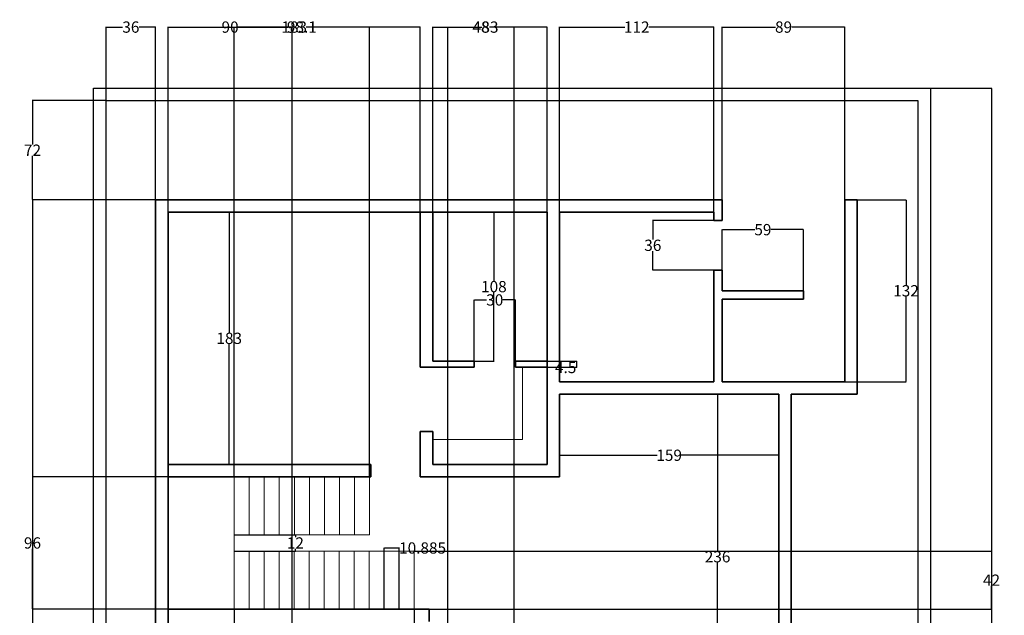
# Model space of a CAD drawing. Units: inches. Extents: x -254 to 1961, y 86 to 3025.
# Tile 6 of 6: x 1247 to 1961, y 2593 to 3025. Entities that reach past the tile are written whole.
import ezdxf

# ---------------------------------------------------------------- set-up
doc = ezdxf.new("R2010")
doc.units = ezdxf.units.IN
doc.header["$MEASUREMENT"] = 0
for name, color, linetype, lineweight in [('A-ANNO-DIMS', 2, 'Continuous', 18), ('C-SITE-WALL', 8, 'Continuous', 30), ('KITCHEN', 9, 'Continuous', 18), ('STAIRCASE', 212, 'Continuous', 18), ('WALLS', 255, 'Continuous', 35)]:
    doc.layers.add(name, color=color, linetype=linetype, lineweight=lineweight)
doc.styles.get("Standard").update_dxf_attribs({"font": 'arial.ttf'})
doc.dimstyles.get("Standard").update_dxf_attribs({"dimtxt": 8.18, "dimasz": 0.18, "dimexe": 0.18, "dimexo": 0.0625, "dimgap": 0.09, "dimtad": 0, "dimtih": 1, "dimtoh": 1, "dimdec": 1, "dimzin": 0, "dimdsep": 46, "dimlunit": 3, "dimtxsty": 'Standard', "dimcen": 0.09, "dimadec": 0, "dimazin": 0, "dimtfac": 1, "dimtdec": 1, "dimtofl": 0, "dimtmove": 0, "dimatfit": 3, "dimfxl": 1, "dimtolj": 1, "dimtzin": 0, "dimarcsym": 0})

# ---------------------------------------------------------------- blocks, each defined once
blk = doc.blocks.new('*D72')
at = {"layer": 'A-ANNO-DIMS', "color": 0, "lineweight": -2, "transparency": 16777216}
for p, q in [((1907.43, 2975.46), (1951.9, 2975.46)), ((1951.72, 2975.28), (1951.72, 2539.72)), ((1951.72, 2095.64), (1951.72, 2531.19)), ((1907.43, 2095.46), (1951.9, 2095.46))]:
    blk.add_line(p, q, dxfattribs=at)
at = {"layer": 'A-ANNO-DIMS', "color": 0, "transparency": 16777216}
for points in [[(1951.69, 2975.28), (1951.75, 2975.28), (1951.72, 2975.46)], [(1951.69, 2095.64), (1951.75, 2095.64), (1951.72, 2095.46)]]:
    blk.add_solid(points, dxfattribs=at)
at = {"layer": 'Defpoints', "color": 0, "transparency": 16777216}
for p in [(1907.37, 2975.46), (1951.72, 2975.46), (1907.37, 2095.46)]:
    blk.add_point(p, dxfattribs=at)
at = {"layer": 'A-ANNO-DIMS', "color": 0, "transparency": 16777216, "insert": (1951.72, 2535.46), "char_height": 8.18, "attachment_point": 5}
blk.add_mtext('\\A1;880', dxfattribs=at)
blk = doc.blocks.new('*D74')
at = {"layer": 'A-ANNO-DIMS', "color": 0, "lineweight": -2, "transparency": 16777216}
for p, q in [((1345.31, 2894.46), (1255.84, 2894.46)), ((1256.02, 2894.28), (1256.02, 2521.71)), ((1256.02, 2140.64), (1256.02, 2513.21)), ((1345.31, 2140.46), (1255.84, 2140.46))]:
    blk.add_line(p, q, dxfattribs=at)
at = {"layer": 'A-ANNO-DIMS', "color": 0, "transparency": 16777216}
for points in [[(1255.99, 2894.28), (1256.05, 2894.28), (1256.02, 2894.46)], [(1255.99, 2140.64), (1256.05, 2140.64), (1256.02, 2140.46)]]:
    blk.add_solid(points, dxfattribs=at)
at = {"layer": 'Defpoints', "color": 0, "transparency": 16777216}
for p in [(1256.02, 2894.46), (1345.37, 2894.46), (1345.37, 2140.46)]:
    blk.add_point(p, dxfattribs=at)
at = {"layer": 'A-ANNO-DIMS', "color": 0, "transparency": 16777216, "insert": (1256.02, 2517.46), "char_height": 8.18, "attachment_point": 5}
blk.add_mtext('\\A1;754', dxfattribs=at)
blk = doc.blocks.new('*D75')
at = {"layer": 'A-ANNO-DIMS', "color": 0, "lineweight": -2, "transparency": 16777216}
for p, q in [((1309.37, 2966.52), (1309.37, 3019.99)), ((1309.55, 3019.81), (1321.43, 3019.81)), ((1345.19, 3019.81), (1333.31, 3019.81)), ((1345.37, 2894.52), (1345.37, 3019.99))]:
    blk.add_line(p, q, dxfattribs=at)
at = {"layer": 'A-ANNO-DIMS', "color": 0, "transparency": 16777216}
for points in [[(1309.55, 3019.84), (1309.55, 3019.78), (1309.37, 3019.81)], [(1345.19, 3019.84), (1345.19, 3019.78), (1345.37, 3019.81)]]:
    blk.add_solid(points, dxfattribs=at)
at = {"layer": 'Defpoints', "color": 0, "transparency": 16777216}
for p in [(1345.37, 3019.81), (1309.37, 2966.46), (1345.37, 2894.46)]:
    blk.add_point(p, dxfattribs=at)
at = {"layer": 'A-ANNO-DIMS', "color": 0, "transparency": 16777216, "insert": (1327.37, 3019.81), "char_height": 8.18, "attachment_point": 5}
blk.add_mtext('\\A1;36', dxfattribs=at)
blk = doc.blocks.new('*D76')
at = {"layer": 'A-ANNO-DIMS', "color": 0, "lineweight": -2, "transparency": 16777216}
for p, q in [((1309.31, 2966.46), (1255.84, 2966.46)), ((1256.02, 2966.28), (1256.02, 2934.65)), ((1256.02, 2894.64), (1256.02, 2926.26)), ((1345.31, 2894.46), (1255.84, 2894.46))]:
    blk.add_line(p, q, dxfattribs=at)
at = {"layer": 'A-ANNO-DIMS', "color": 0, "transparency": 16777216}
for points in [[(1255.99, 2966.28), (1256.05, 2966.28), (1256.02, 2966.46)], [(1255.99, 2894.64), (1256.05, 2894.64), (1256.02, 2894.46)]]:
    blk.add_solid(points, dxfattribs=at)
at = {"layer": 'Defpoints', "color": 0, "transparency": 16777216}
for p in [(1309.37, 2966.46), (1256.02, 2894.46), (1345.37, 2894.46)]:
    blk.add_point(p, dxfattribs=at)
at = {"layer": 'A-ANNO-DIMS', "color": 0, "transparency": 16777216, "insert": (1256.02, 2930.46), "char_height": 8.18, "attachment_point": 5}
blk.add_mtext('\\A1;72', dxfattribs=at)
blk = doc.blocks.new('*D77')
at = {"layer": 'A-ANNO-DIMS', "color": 0, "lineweight": -2, "transparency": 16777216}
for p, q in [((1354.37, 2885.52), (1354.37, 3019.99)), ((1354.55, 3019.81), (1437.13, 3019.81)), ((1537.19, 3019.81), (1454.61, 3019.81)), ((1537.37, 2885.52), (1537.37, 3019.99))]:
    blk.add_line(p, q, dxfattribs=at)
at = {"layer": 'A-ANNO-DIMS', "color": 0, "transparency": 16777216}
for points in [[(1354.55, 3019.84), (1354.55, 3019.78), (1354.37, 3019.81)], [(1537.19, 3019.84), (1537.19, 3019.78), (1537.37, 3019.81)]]:
    blk.add_solid(points, dxfattribs=at)
at = {"layer": 'Defpoints', "color": 0, "transparency": 16777216}
for p in [(1537.37, 3019.81), (1354.37, 2885.46), (1537.37, 2885.46)]:
    blk.add_point(p, dxfattribs=at)
at = {"layer": 'A-ANNO-DIMS', "color": 0, "transparency": 16777216, "insert": (1445.87, 3019.81), "char_height": 8.18, "attachment_point": 5}
blk.add_mtext('\\A1;183', dxfattribs=at)
blk = doc.blocks.new('*D78')
at = {"layer": 'A-ANNO-DIMS', "color": 0, "lineweight": -2, "transparency": 16777216}
for p, q in [((1546.37, 2885.52), (1546.37, 3019.99)), ((1546.55, 3019.81), (1581.91, 3019.81)), ((1629.19, 3019.81), (1593.82, 3019.81)), ((1629.37, 2885.52), (1629.37, 3019.99))]:
    blk.add_line(p, q, dxfattribs=at)
at = {"layer": 'A-ANNO-DIMS', "color": 0, "transparency": 16777216}
for points in [[(1546.55, 3019.84), (1546.55, 3019.78), (1546.37, 3019.81)], [(1629.19, 3019.84), (1629.19, 3019.78), (1629.37, 3019.81)]]:
    blk.add_solid(points, dxfattribs=at)
at = {"layer": 'Defpoints', "color": 0, "transparency": 16777216}
for p in [(1629.37, 3019.81), (1546.37, 2885.46), (1629.37, 2885.46)]:
    blk.add_point(p, dxfattribs=at)
at = {"layer": 'A-ANNO-DIMS', "color": 0, "transparency": 16777216, "insert": (1587.87, 3019.81), "char_height": 8.18, "attachment_point": 5}
blk.add_mtext('\\A1;83', dxfattribs=at)
blk = doc.blocks.new('*D79')
at = {"layer": 'A-ANNO-DIMS', "color": 0, "lineweight": -2, "transparency": 16777216}
for p, q in [((1638.37, 2885.52), (1638.37, 3019.99)), ((1638.55, 3019.81), (1685.67, 3019.81)), ((1750.19, 3019.81), (1703.07, 3019.81)), ((1750.37, 2885.52), (1750.37, 3019.99))]:
    blk.add_line(p, q, dxfattribs=at)
at = {"layer": 'A-ANNO-DIMS', "color": 0, "transparency": 16777216}
for points in [[(1638.55, 3019.84), (1638.55, 3019.78), (1638.37, 3019.81)], [(1750.19, 3019.84), (1750.19, 3019.78), (1750.37, 3019.81)]]:
    blk.add_solid(points, dxfattribs=at)
at = {"layer": 'Defpoints', "color": 0, "transparency": 16777216}
for p in [(1750.37, 3019.81), (1638.37, 2885.46), (1750.37, 2885.46)]:
    blk.add_point(p, dxfattribs=at)
at = {"layer": 'A-ANNO-DIMS', "color": 0, "transparency": 16777216, "insert": (1694.37, 3019.81), "char_height": 8.18, "attachment_point": 5}
blk.add_mtext('\\A1;112', dxfattribs=at)
blk = doc.blocks.new('*D80')
at = {"layer": 'A-ANNO-DIMS', "color": 0, "lineweight": -2, "transparency": 16777216}
for p, q in [((1756.37, 2894.52), (1756.37, 3019.99)), ((1756.55, 3019.81), (1794.91, 3019.81)), ((1845.19, 3019.81), (1806.83, 3019.81)), ((1845.37, 2894.52), (1845.37, 3019.99))]:
    blk.add_line(p, q, dxfattribs=at)
at = {"layer": 'A-ANNO-DIMS', "color": 0, "transparency": 16777216}
for points in [[(1756.55, 3019.84), (1756.55, 3019.78), (1756.37, 3019.81)], [(1845.19, 3019.84), (1845.19, 3019.78), (1845.37, 3019.81)]]:
    blk.add_solid(points, dxfattribs=at)
at = {"layer": 'Defpoints', "color": 0, "transparency": 16777216}
for p in [(1845.37, 3019.81), (1756.37, 2894.46), (1845.37, 2894.46)]:
    blk.add_point(p, dxfattribs=at)
at = {"layer": 'A-ANNO-DIMS', "color": 0, "transparency": 16777216, "insert": (1800.87, 3019.81), "char_height": 8.18, "attachment_point": 5}
blk.add_mtext('\\A1;89', dxfattribs=at)
blk = doc.blocks.new('*D81')
at = {"layer": 'A-ANNO-DIMS', "color": 0, "lineweight": -2, "transparency": 16777216}
for p, q in [((1354.43, 2885.46), (1398.9, 2885.46)), ((1398.72, 2885.28), (1398.72, 2798.22)), ((1398.72, 2702.64), (1398.72, 2789.69)), ((1354.43, 2702.46), (1398.9, 2702.46))]:
    blk.add_line(p, q, dxfattribs=at)
at = {"layer": 'A-ANNO-DIMS', "color": 0, "transparency": 16777216}
for points in [[(1398.69, 2885.28), (1398.75, 2885.28), (1398.72, 2885.46)], [(1398.69, 2702.64), (1398.75, 2702.64), (1398.72, 2702.46)]]:
    blk.add_solid(points, dxfattribs=at)
at = {"layer": 'Defpoints', "color": 0, "transparency": 16777216}
for p in [(1354.37, 2885.46), (1354.37, 2702.46), (1398.72, 2702.46)]:
    blk.add_point(p, dxfattribs=at)
at = {"layer": 'A-ANNO-DIMS', "color": 0, "transparency": 16777216, "insert": (1398.72, 2793.96), "char_height": 8.18, "attachment_point": 5}
blk.add_mtext('\\A1;183', dxfattribs=at)
blk = doc.blocks.new('*D82')
at = {"layer": 'A-ANNO-DIMS', "color": 0, "lineweight": -2, "transparency": 16777216}
for p, q in [((1546.43, 2885.46), (1590.9, 2885.46)), ((1590.72, 2885.28), (1590.72, 2835.72)), ((1590.72, 2777.64), (1590.72, 2827.19)), ((1546.43, 2777.46), (1590.9, 2777.46))]:
    blk.add_line(p, q, dxfattribs=at)
at = {"layer": 'A-ANNO-DIMS', "color": 0, "transparency": 16777216}
for points in [[(1590.69, 2885.28), (1590.75, 2885.28), (1590.72, 2885.46)], [(1590.69, 2777.64), (1590.75, 2777.64), (1590.72, 2777.46)]]:
    blk.add_solid(points, dxfattribs=at)
at = {"layer": 'Defpoints', "color": 0, "transparency": 16777216}
for p in [(1546.37, 2885.46), (1546.37, 2777.46), (1590.72, 2777.46)]:
    blk.add_point(p, dxfattribs=at)
at = {"layer": 'A-ANNO-DIMS', "color": 0, "transparency": 16777216, "insert": (1590.72, 2831.46), "char_height": 8.18, "attachment_point": 5}
blk.add_mtext('\\A1;108', dxfattribs=at)
blk = doc.blocks.new('*D83')
at = {"layer": 'A-ANNO-DIMS', "color": 0, "lineweight": -2, "transparency": 16777216}
for p, q in [((1576.37, 2777.52), (1576.37, 2821.99)), ((1576.55, 2821.81), (1585.44, 2821.81)), ((1606.19, 2821.81), (1597.3, 2821.81)), ((1606.37, 2777.52), (1606.37, 2821.99))]:
    blk.add_line(p, q, dxfattribs=at)
at = {"layer": 'A-ANNO-DIMS', "color": 0, "transparency": 16777216}
for points in [[(1576.55, 2821.84), (1576.55, 2821.78), (1576.37, 2821.81)], [(1606.19, 2821.84), (1606.19, 2821.78), (1606.37, 2821.81)]]:
    blk.add_solid(points, dxfattribs=at)
at = {"layer": 'Defpoints', "color": 0, "transparency": 16777216}
for p in [(1606.37, 2821.81), (1576.37, 2777.46), (1606.37, 2777.46)]:
    blk.add_point(p, dxfattribs=at)
at = {"layer": 'A-ANNO-DIMS', "color": 0, "transparency": 16777216, "insert": (1591.37, 2821.81), "char_height": 8.18, "attachment_point": 5}
blk.add_mtext('\\A1;30', dxfattribs=at)
blk = doc.blocks.new('*D84')
at = {"layer": 'A-ANNO-DIMS', "color": 0, "lineweight": -2, "transparency": 16777216}
for p, q in [((1750.31, 2879.46), (1705.84, 2879.46)), ((1706.02, 2879.28), (1706.02, 2865.72)), ((1706.02, 2843.64), (1706.02, 2857.19)), ((1750.31, 2843.46), (1705.84, 2843.46))]:
    blk.add_line(p, q, dxfattribs=at)
at = {"layer": 'A-ANNO-DIMS', "color": 0, "transparency": 16777216}
for points in [[(1705.99, 2879.28), (1706.05, 2879.28), (1706.02, 2879.46)], [(1705.99, 2843.64), (1706.05, 2843.64), (1706.02, 2843.46)]]:
    blk.add_solid(points, dxfattribs=at)
at = {"layer": 'Defpoints', "color": 0, "transparency": 16777216}
for p in [(1706.02, 2879.46), (1750.37, 2879.46), (1750.37, 2843.46)]:
    blk.add_point(p, dxfattribs=at)
at = {"layer": 'A-ANNO-DIMS', "color": 0, "transparency": 16777216, "insert": (1706.02, 2861.46), "char_height": 8.18, "attachment_point": 5}
blk.add_mtext('\\A1;36', dxfattribs=at)
blk = doc.blocks.new('*D85')
at = {"layer": 'A-ANNO-DIMS', "color": 0, "lineweight": -2, "transparency": 16777216}
for p, q in [((1845.43, 2894.46), (1889.9, 2894.46)), ((1889.72, 2894.28), (1889.72, 2832.72)), ((1889.72, 2762.64), (1889.72, 2824.19)), ((1845.43, 2762.46), (1889.9, 2762.46))]:
    blk.add_line(p, q, dxfattribs=at)
at = {"layer": 'A-ANNO-DIMS', "color": 0, "transparency": 16777216}
for points in [[(1889.69, 2894.28), (1889.75, 2894.28), (1889.72, 2894.46)], [(1889.69, 2762.64), (1889.75, 2762.64), (1889.72, 2762.46)]]:
    blk.add_solid(points, dxfattribs=at)
at = {"layer": 'Defpoints', "color": 0, "transparency": 16777216}
for p in [(1845.37, 2894.46), (1845.37, 2762.46), (1889.72, 2762.46)]:
    blk.add_point(p, dxfattribs=at)
at = {"layer": 'A-ANNO-DIMS', "color": 0, "transparency": 16777216, "insert": (1889.72, 2828.46), "char_height": 8.18, "attachment_point": 5}
blk.add_mtext('\\A1;132', dxfattribs=at)
blk = doc.blocks.new('*D86')
at = {"layer": 'A-ANNO-DIMS', "color": 0, "lineweight": -2, "transparency": 16777216}
for p, q in [((1354.31, 2693.46), (1255.84, 2693.46)), ((1256.02, 2693.28), (1256.02, 2649.72)), ((1256.02, 2597.64), (1256.02, 2641.19)), ((1354.31, 2597.46), (1255.84, 2597.46))]:
    blk.add_line(p, q, dxfattribs=at)
at = {"layer": 'A-ANNO-DIMS', "color": 0, "transparency": 16777216}
for points in [[(1255.99, 2693.28), (1256.05, 2693.28), (1256.02, 2693.46)], [(1255.99, 2597.64), (1256.05, 2597.64), (1256.02, 2597.46)]]:
    blk.add_solid(points, dxfattribs=at)
at = {"layer": 'Defpoints', "color": 0, "transparency": 16777216}
for p in [(1354.37, 2693.46), (1256.02, 2597.46), (1354.37, 2597.46)]:
    blk.add_point(p, dxfattribs=at)
at = {"layer": 'A-ANNO-DIMS', "color": 0, "transparency": 16777216, "insert": (1256.02, 2645.46), "char_height": 8.18, "attachment_point": 5}
blk.add_mtext('\\A1;96', dxfattribs=at)
blk = doc.blocks.new('*D87')
at = {"layer": 'A-ANNO-DIMS', "color": 0, "lineweight": -2, "transparency": 16777216}
for p, q in [((1797.31, 2753.46), (1752.84, 2753.46)), ((1753.02, 2753.28), (1753.02, 2639.72)), ((1753.02, 2517.64), (1753.02, 2631.19)), ((1797.31, 2517.46), (1752.84, 2517.46))]:
    blk.add_line(p, q, dxfattribs=at)
at = {"layer": 'A-ANNO-DIMS', "color": 0, "transparency": 16777216}
for points in [[(1752.99, 2753.28), (1753.05, 2753.28), (1753.02, 2753.46)], [(1752.99, 2517.64), (1753.05, 2517.64), (1753.02, 2517.46)]]:
    blk.add_solid(points, dxfattribs=at)
at = {"layer": 'Defpoints', "color": 0, "transparency": 16777216}
for p in [(1753.02, 2753.46), (1797.37, 2753.46), (1797.37, 2517.46)]:
    blk.add_point(p, dxfattribs=at)
at = {"layer": 'A-ANNO-DIMS', "color": 0, "transparency": 16777216, "insert": (1753.02, 2635.46), "char_height": 8.18, "attachment_point": 5}
blk.add_mtext('\\A1;236', dxfattribs=at)
blk = doc.blocks.new('*D93')
at = {"layer": 'A-ANNO-DIMS', "color": 0, "lineweight": -2, "transparency": 16777216}
for p, q in [((1402.37, 2597.39), (1402.37, 2050.93)), ((1532.98, 2597.39), (1532.98, 2050.93)), ((1402.55, 2051.11), (1451.03, 2051.11)), ((1532.8, 2051.11), (1484.32, 2051.11))]:
    blk.add_line(p, q, dxfattribs=at)
at = {"layer": 'A-ANNO-DIMS', "color": 0, "transparency": 16777216}
for points in [[(1402.55, 2051.14), (1402.55, 2051.08), (1402.37, 2051.11)], [(1532.8, 2051.14), (1532.8, 2051.08), (1532.98, 2051.11)]]:
    blk.add_solid(points, dxfattribs=at)
at = {"layer": 'Defpoints', "color": 0, "transparency": 16777216}
for p in [(1402.37, 2597.46), (1532.98, 2597.46), (1532.98, 2051.11)]:
    blk.add_point(p, dxfattribs=at)
at = {"layer": 'A-ANNO-DIMS', "color": 0, "transparency": 16777216, "insert": (1467.68, 2051.11), "char_height": 8.18, "attachment_point": 5}
blk.add_mtext('\\A1;130.62', dxfattribs=at)
blk = doc.blocks.new('*D94')
at = {"layer": 'A-ANNO-DIMS', "color": 0, "lineweight": -2, "transparency": 16777216}
for p, q in [((1354.37, 2597.39), (1354.37, 2050.93)), ((1402.37, 2597.39), (1402.37, 2050.93)), ((1354.55, 2051.11), (1372.25, 2051.11)), ((1402.19, 2051.11), (1384.49, 2051.11))]:
    blk.add_line(p, q, dxfattribs=at)
at = {"layer": 'A-ANNO-DIMS', "color": 0, "transparency": 16777216}
for points in [[(1354.55, 2051.14), (1354.55, 2051.08), (1354.37, 2051.11)], [(1402.19, 2051.14), (1402.19, 2051.08), (1402.37, 2051.11)]]:
    blk.add_solid(points, dxfattribs=at)
at = {"layer": 'Defpoints', "color": 0, "transparency": 16777216}
for p in [(1354.37, 2597.46), (1402.37, 2597.46), (1402.37, 2051.11)]:
    blk.add_point(p, dxfattribs=at)
at = {"layer": 'A-ANNO-DIMS', "color": 0, "transparency": 16777216, "insert": (1378.37, 2051.11), "char_height": 8.18, "attachment_point": 5}
blk.add_mtext('\\A1;48', dxfattribs=at)
blk = doc.blocks.new('*D95')
at = {"layer": 'A-ANNO-DIMS', "color": 0, "lineweight": -2, "transparency": 16777216}
for p, q in [((1402.37, 2693.52), (1402.37, 3019.99)), ((1402.55, 3019.81), (1441.49, 3019.81)), ((1500.29, 3019.81), (1461.34, 3019.81)), ((1500.47, 2693.52), (1500.47, 3019.99))]:
    blk.add_line(p, q, dxfattribs=at)
at = {"layer": 'A-ANNO-DIMS', "color": 0, "transparency": 16777216}
for points in [[(1402.55, 3019.84), (1402.55, 3019.78), (1402.37, 3019.81)], [(1500.29, 3019.84), (1500.29, 3019.78), (1500.47, 3019.81)]]:
    blk.add_solid(points, dxfattribs=at)
at = {"layer": 'Defpoints', "color": 0, "transparency": 16777216}
for p in [(1500.47, 3019.81), (1402.37, 2693.46), (1500.47, 2693.46)]:
    blk.add_point(p, dxfattribs=at)
at = {"layer": 'A-ANNO-DIMS', "color": 0, "transparency": 16777216, "insert": (1451.42, 3019.81), "char_height": 8.18, "attachment_point": 5}
blk.add_mtext('\\A1;98.1', dxfattribs=at)
blk = doc.blocks.new('*D96')
at = {"layer": 'A-ANNO-DIMS', "color": 0, "lineweight": -2, "transparency": 16777216}
for p, q in [((1511.22, 2597.52), (1511.22, 2641.99)), ((1511.4, 2641.81), (1521.92, 2641.81)), ((1522.1, 2597.52), (1522.1, 2641.99)), ((1522.1, 2641.81), (1522.28, 2641.81))]:
    blk.add_line(p, q, dxfattribs=at)
at = {"layer": 'A-ANNO-DIMS', "color": 0, "transparency": 16777216}
for points in [[(1511.4, 2641.84), (1511.4, 2641.78), (1511.22, 2641.81)], [(1521.92, 2641.84), (1521.92, 2641.78), (1522.1, 2641.81)]]:
    blk.add_solid(points, dxfattribs=at)
at = {"layer": 'Defpoints', "color": 0, "transparency": 16777216}
for p in [(1522.1, 2641.81), (1511.22, 2597.46), (1522.1, 2597.46)]:
    blk.add_point(p, dxfattribs=at)
at = {"layer": 'A-ANNO-DIMS', "color": 0, "transparency": 16777216, "insert": (1539, 2641.81), "char_height": 8.18, "attachment_point": 5}
blk.add_mtext('\\A1;10.885', dxfattribs=at)
blk = doc.blocks.new('*D97')
at = {"layer": 'A-ANNO-DIMS', "color": 0, "lineweight": -2, "transparency": 16777216}
for p, q in [((1533.05, 2639.46), (1951.9, 2639.46)), ((1951.72, 2639.28), (1951.72, 2622.65)), ((1951.72, 2597.64), (1951.72, 2614.26)), ((1533.05, 2597.46), (1951.9, 2597.46))]:
    blk.add_line(p, q, dxfattribs=at)
at = {"layer": 'A-ANNO-DIMS', "color": 0, "transparency": 16777216}
for points in [[(1951.69, 2639.28), (1951.75, 2639.28), (1951.72, 2639.46)], [(1951.69, 2597.64), (1951.75, 2597.64), (1951.72, 2597.46)]]:
    blk.add_solid(points, dxfattribs=at)
at = {"layer": 'Defpoints', "color": 0, "transparency": 16777216}
for p in [(1532.98, 2639.46), (1951.72, 2639.46), (1532.98, 2597.46)]:
    blk.add_point(p, dxfattribs=at)
at = {"layer": 'A-ANNO-DIMS', "color": 0, "transparency": 16777216, "insert": (1951.72, 2618.46), "char_height": 8.18, "attachment_point": 5}
blk.add_mtext('\\A1;42', dxfattribs=at)
blk = doc.blocks.new('*D98')
at = {"layer": 'A-ANNO-DIMS', "color": 0, "lineweight": -2, "transparency": 16777216}
for p, q in [((1402.43, 2651.46), (1446.9, 2651.46)), ((1446.72, 2651.28), (1446.72, 2649.65)), ((1402.43, 2639.46), (1446.9, 2639.46)), ((1446.72, 2639.64), (1446.72, 2641.26))]:
    blk.add_line(p, q, dxfattribs=at)
at = {"layer": 'A-ANNO-DIMS', "color": 0, "transparency": 16777216}
for points in [[(1446.69, 2651.28), (1446.75, 2651.28), (1446.72, 2651.46)], [(1446.69, 2639.64), (1446.75, 2639.64), (1446.72, 2639.46)]]:
    blk.add_solid(points, dxfattribs=at)
at = {"layer": 'Defpoints', "color": 0, "transparency": 16777216}
for p in [(1402.37, 2651.46), (1402.37, 2639.46), (1446.72, 2639.46)]:
    blk.add_point(p, dxfattribs=at)
at = {"layer": 'A-ANNO-DIMS', "color": 0, "transparency": 16777216, "insert": (1446.72, 2645.46), "char_height": 8.18, "attachment_point": 5}
blk.add_mtext('\\A1;12', dxfattribs=at)
blk = doc.blocks.new('*D101')
at = {"layer": 'A-ANNO-DIMS', "color": 0, "lineweight": -2, "transparency": 16777216}
for p, q in [((1606.43, 2777.46), (1650.9, 2777.46)), ((1606.43, 2772.96), (1650.9, 2772.96)), ((1650.72, 2772.78), (1650.54, 2772.78)), ((1650.72, 2777.28), (1650.72, 2773.14)), ((1650.72, 2772.96), (1650.72, 2772.78))]:
    blk.add_line(p, q, dxfattribs=at)
at = {"layer": 'A-ANNO-DIMS', "color": 0, "transparency": 16777216}
for points in [[(1650.69, 2777.28), (1650.75, 2777.28), (1650.72, 2777.46)], [(1650.69, 2773.14), (1650.75, 2773.14), (1650.72, 2772.96)]]:
    blk.add_solid(points, dxfattribs=at)
at = {"layer": 'Defpoints', "color": 0, "transparency": 16777216}
for p in [(1606.37, 2777.46), (1606.37, 2772.96), (1650.72, 2772.96)]:
    blk.add_point(p, dxfattribs=at)
at = {"layer": 'A-ANNO-DIMS', "color": 0, "transparency": 16777216, "insert": (1642.81, 2772.78), "char_height": 8.18, "attachment_point": 5}
blk.add_mtext('\\A1;4.5', dxfattribs=at)
blk = doc.blocks.new('*D102')
at = {"layer": 'A-ANNO-DIMS', "color": 0, "lineweight": -2, "transparency": 16777216}
for p, q in [((1756.37, 2828.52), (1756.37, 2872.99)), ((1756.55, 2872.81), (1779.91, 2872.81)), ((1815.19, 2872.81), (1791.83, 2872.81)), ((1815.37, 2828.52), (1815.37, 2872.99))]:
    blk.add_line(p, q, dxfattribs=at)
at = {"layer": 'A-ANNO-DIMS', "color": 0, "transparency": 16777216}
for points in [[(1756.55, 2872.84), (1756.55, 2872.78), (1756.37, 2872.81)], [(1815.19, 2872.84), (1815.19, 2872.78), (1815.37, 2872.81)]]:
    blk.add_solid(points, dxfattribs=at)
at = {"layer": 'Defpoints', "color": 0, "transparency": 16777216}
for p in [(1815.37, 2872.81), (1756.37, 2828.46), (1815.37, 2828.46)]:
    blk.add_point(p, dxfattribs=at)
at = {"layer": 'A-ANNO-DIMS', "color": 0, "transparency": 16777216, "insert": (1785.87, 2872.81), "char_height": 8.18, "attachment_point": 5}
blk.add_mtext('\\A1;59', dxfattribs=at)
blk = doc.blocks.new('*D103')
at = {"layer": 'A-ANNO-DIMS', "color": 0, "lineweight": -2, "transparency": 16777216}
for p, q in [((1638.37, 2753.39), (1638.37, 2708.93)), ((1797.37, 2753.39), (1797.37, 2708.93)), ((1638.55, 2709.11), (1709.12, 2709.11)), ((1797.19, 2709.11), (1726.62, 2709.11))]:
    blk.add_line(p, q, dxfattribs=at)
at = {"layer": 'A-ANNO-DIMS', "color": 0, "transparency": 16777216}
for points in [[(1638.55, 2709.14), (1638.55, 2709.08), (1638.37, 2709.11)], [(1797.19, 2709.14), (1797.19, 2709.08), (1797.37, 2709.11)]]:
    blk.add_solid(points, dxfattribs=at)
at = {"layer": 'Defpoints', "color": 0, "transparency": 16777216}
for p in [(1638.37, 2753.46), (1797.37, 2753.46), (1638.37, 2709.11)]:
    blk.add_point(p, dxfattribs=at)
at = {"layer": 'A-ANNO-DIMS', "color": 0, "transparency": 16777216, "insert": (1717.87, 2709.11), "char_height": 8.18, "attachment_point": 5}
blk.add_mtext('\\A1;159', dxfattribs=at)
blk = doc.blocks.new('*D104')
at = {"layer": 'A-ANNO-DIMS', "color": 0, "lineweight": -2, "transparency": 16777216}
for p, q in [((1354.37, 2322.52), (1354.37, 3019.99)), ((1354.55, 3019.81), (1393.43, 3019.81)), ((1444.19, 3019.81), (1405.3, 3019.81)), ((1444.37, 2322.52), (1444.37, 3019.99))]:
    blk.add_line(p, q, dxfattribs=at)
at = {"layer": 'A-ANNO-DIMS', "color": 0, "transparency": 16777216}
for points in [[(1354.55, 3019.84), (1354.55, 3019.78), (1354.37, 3019.81)], [(1444.19, 3019.84), (1444.19, 3019.78), (1444.37, 3019.81)]]:
    blk.add_solid(points, dxfattribs=at)
at = {"layer": 'Defpoints', "color": 0, "transparency": 16777216}
for p in [(1444.37, 3019.81), (1354.37, 2322.46), (1444.37, 2322.46)]:
    blk.add_point(p, dxfattribs=at)
at = {"layer": 'A-ANNO-DIMS', "color": 0, "transparency": 16777216, "insert": (1399.37, 3019.81), "char_height": 8.18, "attachment_point": 5}
blk.add_mtext('\\A1;90', dxfattribs=at)
blk = doc.blocks.new('*D111')
at = {"layer": 'A-ANNO-DIMS', "color": 0, "lineweight": -2, "transparency": 16777216}
for p, q in [((1557.37, 2221.52), (1557.37, 3019.99)), ((1557.55, 3019.81), (1575.25, 3019.81)), ((1605.19, 3019.81), (1587.49, 3019.81)), ((1605.37, 2173.52), (1605.37, 3019.99))]:
    blk.add_line(p, q, dxfattribs=at)
at = {"layer": 'A-ANNO-DIMS', "color": 0, "transparency": 16777216}
for points in [[(1557.55, 3019.84), (1557.55, 3019.78), (1557.37, 3019.81)], [(1605.19, 3019.84), (1605.19, 3019.78), (1605.37, 3019.81)]]:
    blk.add_solid(points, dxfattribs=at)
at = {"layer": 'Defpoints', "color": 0, "transparency": 16777216}
for p in [(1605.37, 3019.81), (1557.37, 2221.46), (1605.37, 2173.46)]:
    blk.add_point(p, dxfattribs=at)
at = {"layer": 'A-ANNO-DIMS', "color": 0, "transparency": 16777216, "insert": (1581.37, 3019.81), "char_height": 8.18, "attachment_point": 5}
blk.add_mtext('\\A1;48', dxfattribs=at)

msp = doc.modelspace()

# ---------------------------------------------------------------- linework, layer by layer
at = {"layer": 'C-SITE-WALL'}
for points in [[(1300.3694, 2975.4553), (1907.3694, 2975.4553), (1907.3694, 2095.4553), (1300.3694, 2095.4553)], [(1309.3694, 2966.4553), (1898.3694, 2966.4553), (1898.3694, 2104.4553), (1309.3694, 2104.4553)]]:
    msp.add_lwpolyline(points, close=True, dxfattribs=at)
at = {"layer": 'KITCHEN'}
for p, q in [((1611.3694, 2720.4553), (1611.3694, 2772.9553)), ((1546.3694, 2720.4553), (1611.3694, 2720.4553))]:
    msp.add_line(p, q, dxfattribs=at)
at = {"layer": 'STAIRCASE'}
for p, q in [((1413.2694, 2651.4553), (1413.2694, 2693.4553)), ((1424.1694, 2651.4553), (1424.1694, 2693.4553)), ((1435.0694, 2651.4553), (1435.0694, 2693.4553)), ((1445.9694, 2651.4553), (1445.9694, 2693.4553)), ((1456.8694, 2651.4553), (1456.8694, 2693.4553)), ((1467.7694, 2651.4553), (1467.7694, 2693.4553)), ((1478.6694, 2651.4553), (1478.6694, 2693.4553)), ((1489.5694, 2651.4553), (1489.5694, 2693.4553)), ((1413.254, 2597.4553), (1413.254, 2639.4553)), ((1424.1386, 2597.4553), (1424.1386, 2639.4553)), ((1435.0232, 2597.4553), (1435.0232, 2639.4553)), ((1445.9078, 2597.4553), (1445.9078, 2639.4553)), ((1456.7925, 2597.4553), (1456.7925, 2639.4553)), ((1467.6771, 2597.4553), (1467.6771, 2639.4553)), ((1478.5617, 2597.4553), (1478.5617, 2639.4553)), ((1489.4463, 2597.4553), (1489.4463, 2639.4553)), ((1500.3309, 2597.4553), (1500.3309, 2639.4553)), ((1511.2155, 2597.4553), (1511.2155, 2639.4553)), ((1522.1001, 2597.4553), (1522.1001, 2639.4553))]:
    msp.add_line(p, q, dxfattribs=at)
msp.add_lwpolyline([(1500.4694, 2693.4553), (1500.4694, 2651.4553), (1402.3694, 2651.4553), (1402.3694, 2693.4553), (1402.3694, 2597.4553), (1402.3694, 2639.4553), (1532.9848, 2639.4553), (1532.9848, 2597.4553), (1354.3694, 2597.4553), (1354.3694, 2693.4553)], close=True, dxfattribs=at)
at = {"layer": 'WALLS'}
for p, q in [((1345.3694, 2508.4553), (1345.3694, 2894.4553)), ((1345.3694, 2894.4553), (1756.3694, 2894.4553)), ((1756.3694, 2879.4553), (1756.3694, 2894.4553)), ((1845.3694, 2762.4553), (1845.3694, 2894.4553)), ((1845.3694, 2894.4553), (1854.3694, 2894.4553)), ((1854.3694, 2753.4553), (1854.3694, 2894.4553)), ((1354.3694, 2597.4553), (1354.3694, 2885.4553)), ((1354.3694, 2885.4553), (1629.3694, 2885.4553)), ((1537.3694, 2772.9553), (1537.3694, 2885.4553)), ((1546.3694, 2777.4553), (1546.3694, 2885.4553)), ((1629.3694, 2702.4553), (1629.3694, 2885.4553)), ((1638.3694, 2762.4553), (1638.3694, 2885.4553)), ((1638.3694, 2885.4553), (1750.3694, 2885.4553)), ((1750.3694, 2879.4553), (1750.3694, 2885.4553)), ((1750.3694, 2879.4553), (1756.3694, 2879.4553)), ((1750.3694, 2762.4553), (1750.3694, 2843.4553)), ((1750.3694, 2843.4553), (1756.3694, 2843.4553)), ((1756.3694, 2828.4553), (1756.3694, 2843.4553)), ((1756.3694, 2828.4553), (1815.3694, 2828.4553)), ((1756.3694, 2762.4553), (1756.3694, 2822.4553)), ((1756.3694, 2822.4553), (1815.3694, 2822.4553)), ((1815.3694, 2822.4553), (1815.3694, 2828.4553)), ((1537.3694, 2772.9553), (1576.3694, 2772.9553)), ((1546.3694, 2777.4553), (1576.3694, 2777.4553)), ((1576.3694, 2772.9553), (1576.3694, 2777.4553)), ((1606.3694, 2772.9553), (1606.3694, 2777.4553)), ((1606.3694, 2777.4553), (1629.3694, 2777.4553)), ((1606.3694, 2772.9553), (1629.3694, 2772.9553)), ((1638.3694, 2762.4553), (1750.3694, 2762.4553)), ((1756.3694, 2762.4553), (1845.3694, 2762.4553)), ((1638.3694, 2753.4553), (1797.3694, 2753.4553)), ((1638.3694, 2693.4553), (1638.3694, 2753.4553)), ((1797.3694, 2517.4553), (1797.3694, 2753.4553)), ((1806.3694, 2517.4553), (1806.3694, 2753.4553)), ((1806.3694, 2753.4553), (1854.3694, 2753.4553)), ((1537.3694, 2693.4553), (1537.3694, 2726.4553)), ((1537.3694, 2726.4553), (1546.3694, 2726.4553)), ((1546.3694, 2702.4553), (1546.3694, 2726.4553)), ((1354.3694, 2702.4553), (1501.3694, 2702.4553)), ((1501.3694, 2693.4553), (1501.3694, 2702.4553)), ((1546.3694, 2702.4553), (1629.3694, 2702.4553)), ((1354.3694, 2693.4553), (1501.3694, 2693.4553)), ((1537.3694, 2693.4553), (1638.3694, 2693.4553)), ((1354.3694, 2597.4553), (1543.8694, 2597.4553)), ((1543.8694, 2588.4553), (1543.8694, 2597.4553))]:
    msp.add_line(p, q, dxfattribs=at)

# ---------------------------------------------------------------- dimensions: what is measured, and where the dimension line sits
at = {"layer": 'A-ANNO-DIMS'}
for base, p1, p2, override, picture, middle in [((1345.3694, 3019.8053), (1309.3694, 2966.4553), (1345.3694, 2894.4553), {"dimdec": 0, "dimlfac": 1, "dimrnd": 0, "dimzin": 0, "dimdsep": 46, "dimlunit": 2}, '*D75', (1327.3694, 3019.8053)), ((1537.3694, 3019.8053), (1354.3694, 2885.4553), (1537.3694, 2885.4553), {"dimdec": 0, "dimlfac": 1, "dimrnd": 0, "dimzin": 0, "dimdsep": 46, "dimlunit": 2}, '*D77', (1445.8694, 3019.8053)), ((1444.3694, 3019.8053), (1354.3694, 2322.4553), (1444.3694, 2322.4553), {"dimdec": 0, "dimlfac": 1, "dimrnd": 0, "dimzin": 0, "dimdsep": 46, "dimlunit": 2}, '*D104', (1399.3694, 3019.8053)), ((1500.4694, 3019.8053), (1402.3694, 2693.4553), (1500.4694, 2693.4553), {"dimdec": 1, "dimlfac": 1, "dimrnd": 0, "dimzin": 0, "dimdsep": 46, "dimlunit": 2}, '*D95', (1451.4194, 3019.8053)), ((1629.3694, 3019.8053), (1546.3694, 2885.4553), (1629.3694, 2885.4553), {"dimdec": 0, "dimlfac": 1, "dimrnd": 0, "dimzin": 0, "dimdsep": 46, "dimlunit": 2}, '*D78', (1587.8694, 3019.8053)), ((1605.3694, 3019.8053), (1557.3694, 2221.4553), (1605.3694, 2173.4553), {"dimdec": 0, "dimlfac": 1, "dimrnd": 0, "dimzin": 0, "dimdsep": 46, "dimlunit": 2}, '*D111', (1581.3694, 3019.8053)), ((1750.3694, 3019.8053), (1638.3694, 2885.4553), (1750.3694, 2885.4553), {"dimdec": 0, "dimlfac": 1, "dimrnd": 0, "dimzin": 0, "dimdsep": 46, "dimlunit": 2}, '*D79', (1694.3694, 3019.8053)), ((1845.3694, 3019.8053), (1756.3694, 2894.4553), (1845.3694, 2894.4553), {"dimdec": 0, "dimlfac": 1, "dimrnd": 0, "dimzin": 0, "dimdsep": 46, "dimlunit": 2}, '*D80', (1800.8694, 3019.8053)), ((1815.3694, 2872.8053), (1756.3694, 2828.4553), (1815.3694, 2828.4553), {"dimdec": 0, "dimlfac": 1, "dimrnd": 0, "dimzin": 0, "dimdsep": 46, "dimlunit": 2}, '*D102', (1785.8694, 2872.8053)), ((1606.3694, 2821.8053), (1576.3694, 2777.4553), (1606.3694, 2777.4553), {"dimdec": 0, "dimlfac": 1, "dimrnd": 0, "dimzin": 0, "dimdsep": 46, "dimlunit": 2}, '*D83', (1591.3694, 2821.8053)), ((1522.1001, 2641.8053), (1511.2155, 2597.4553), (1522.1001, 2597.4553), {"dimdec": 3, "dimlfac": 1, "dimrnd": 0, "dimzin": 0, "dimdsep": 46, "dimlunit": 2}, '*D96', (1538.9952, 2641.8053)), ((1402.3694, 2051.1053), (1354.3694, 2597.4553), (1402.3694, 2597.4553), {"dimdec": 0, "dimlfac": 1, "dimrnd": 0, "dimzin": 0, "dimdsep": 46, "dimlunit": 2}, '*D94', (1378.3694, 2051.1053)), ((1532.9848, 2051.1053), (1402.3694, 2597.4553), (1532.9848, 2597.4553), {"dimdec": 2, "dimlfac": 1, "dimrnd": 0, "dimzin": 0, "dimdsep": 46, "dimlunit": 2}, '*D93', (1467.6771, 2051.1053))]:
    dim = msp.add_linear_dim(base=base, p1=p1, p2=p2, dimstyle='Standard', override=override, dxfattribs=at)
    dim.commit()
    dim.dimension.update_dxf_attribs({"geometry": picture, "text_midpoint": middle})
for base, p1, p2, angle, override, picture, middle in [((1951.7194, 2975.4553), (1907.3694, 2095.4553), (1907.3694, 2975.4553), 90, {"dimdec": 0, "dimlfac": 1, "dimrnd": 0, "dimzin": 0, "dimdsep": 46, "dimlunit": 2}, '*D72', (1951.7194, 2535.4553)), ((1256.0194, 2894.4553), (1309.3694, 2966.4553), (1345.3694, 2894.4553), 90, {"dimdec": 0, "dimlfac": 1, "dimrnd": 0, "dimzin": 0, "dimdsep": 46, "dimlunit": 2}, '*D76', (1256.0194, 2930.4553)), ((1256.0194, 2894.4553), (1345.3694, 2140.4553), (1345.3694, 2894.4553), 90, {"dimdec": 0, "dimlfac": 1, "dimrnd": 0, "dimzin": 0, "dimdsep": 46, "dimlunit": 2}, '*D74', (1256.0194, 2517.4553)), ((1889.7194, 2762.4553), (1845.3694, 2894.4553), (1845.3694, 2762.4553), 270, {"dimdec": 0, "dimlfac": 1, "dimrnd": 0, "dimzin": 0, "dimdsep": 46, "dimlunit": 2}, '*D85', (1889.7194, 2828.4553)), ((1398.7194, 2702.4553), (1354.3694, 2885.4553), (1354.3694, 2702.4553), 270, {"dimdec": 0, "dimlfac": 1, "dimrnd": 0, "dimzin": 0, "dimdsep": 46, "dimlunit": 2}, '*D81', (1398.7194, 2793.9553)), ((1590.7194, 2777.4553), (1546.3694, 2885.4553), (1546.3694, 2777.4553), 270, {"dimdec": 0, "dimlfac": 1, "dimrnd": 0, "dimzin": 0, "dimdsep": 46, "dimlunit": 2}, '*D82', (1590.7194, 2831.4553)), ((1706.0194, 2879.4553), (1750.3694, 2843.4553), (1750.3694, 2879.4553), 90, {"dimdec": 0, "dimlfac": 1, "dimrnd": 0, "dimzin": 0, "dimdsep": 46, "dimlunit": 2}, '*D84', (1706.0194, 2861.4553)), ((1650.7194, 2772.9553), (1606.3694, 2777.4553), (1606.3694, 2772.9553), 270, {"dimdec": 1, "dimlfac": 1, "dimrnd": 0, "dimzin": 0, "dimdsep": 46, "dimlunit": 2}, '*D101', (1642.8078, 2772.7753)), ((1638.3694, 2709.1053), (1797.3694, 2753.4553), (1638.3694, 2753.4553), 180, {"dimdec": 0, "dimlfac": 1, "dimrnd": 0, "dimzin": 0, "dimdsep": 46, "dimlunit": 2}, '*D103', (1717.8694, 2709.1053)), ((1753.0194, 2753.4553), (1797.3694, 2517.4553), (1797.3694, 2753.4553), 90, {"dimdec": 0, "dimlfac": 1, "dimrnd": 0, "dimzin": 0, "dimdsep": 46, "dimlunit": 2}, '*D87', (1753.0194, 2635.4553)), ((1256.0194, 2597.4553), (1354.3694, 2693.4553), (1354.3694, 2597.4553), 90, {"dimdec": 0, "dimlfac": 1, "dimrnd": 0, "dimzin": 0, "dimdsep": 46, "dimlunit": 2}, '*D86', (1256.0194, 2645.4553)), ((1446.7194, 2639.4553), (1402.3694, 2651.4553), (1402.3694, 2639.4553), 270, {"dimdec": 0, "dimlfac": 1, "dimrnd": 0, "dimzin": 0, "dimdsep": 46, "dimlunit": 2}, '*D98', (1446.7194, 2645.4553)), ((1951.7194, 2639.4553), (1532.9848, 2597.4553), (1532.9848, 2639.4553), 90, {"dimdec": 0, "dimlfac": 1, "dimrnd": 0, "dimzin": 0, "dimdsep": 46, "dimlunit": 2}, '*D97', (1951.7194, 2618.4553))]:
    dim = msp.add_linear_dim(base=base, p1=p1, p2=p2, angle=angle, dimstyle='Standard', override=override, dxfattribs=at)
    dim.commit()
    dim.dimension.update_dxf_attribs({"geometry": picture, "text_midpoint": middle})

doc.saveas('drawing.dxf')
